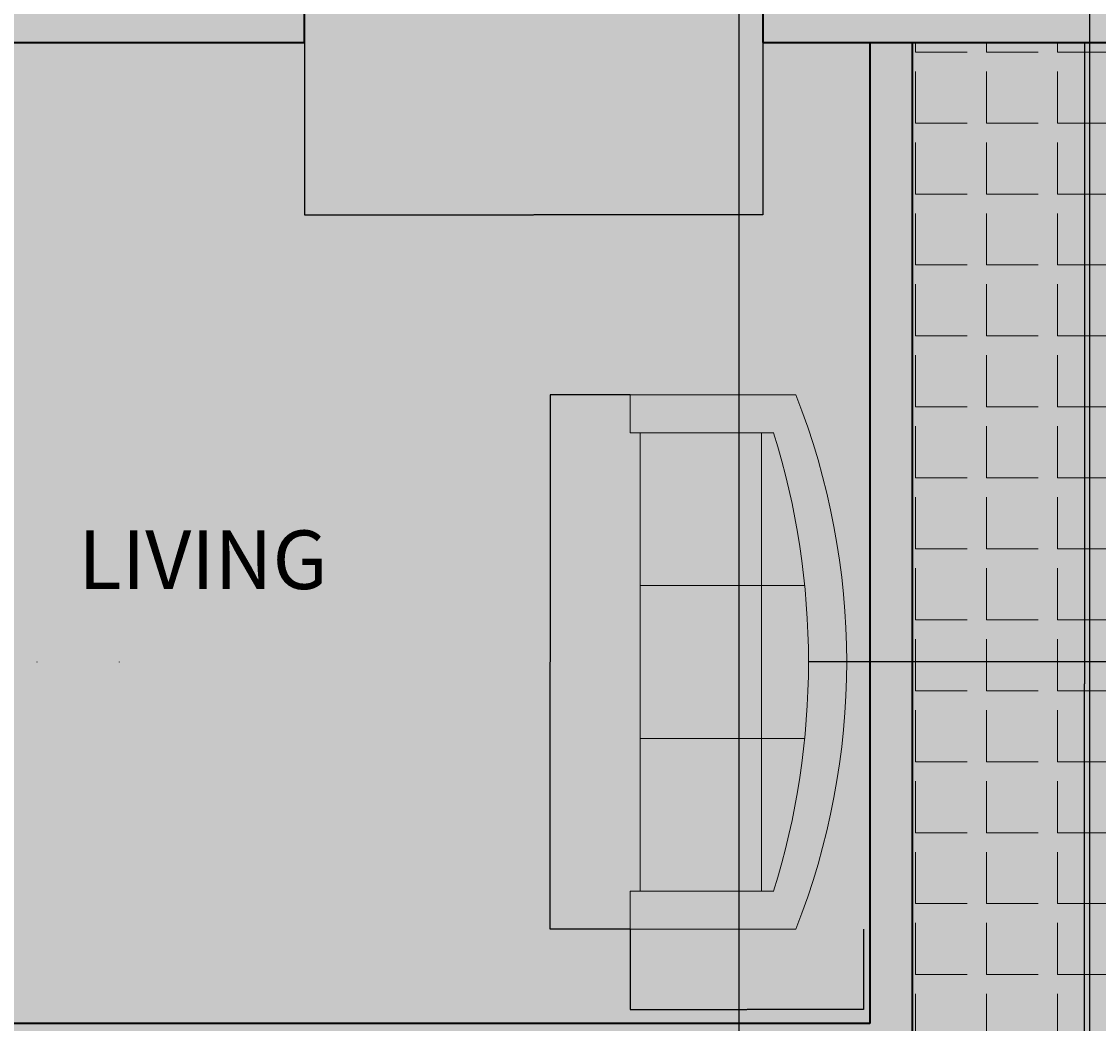
# Model space of a CAD drawing. Units: millimetres. Extents: x 1166 to 16630, y -7192 to 2820.
# Tile 3 of 8: x 2769 to 5842, y -5443 to -2583. Entities that reach past the tile are written whole.
import ezdxf

# ---------------------------------------------------------------- set-up
doc = ezdxf.new("R2010")
doc.units = ezdxf.units.MM
for name, color, linetype, lineweight in [('A-ANNO-DIMS', 2, 'Continuous', 18), ('A-AREA-IDEN', 7, 'Continuous', 18), ('A-FLOR-PATT', 8, 'Continuous', 13), ('A-FURN', 8, 'Continuous', 18), ('A-WALL', 7, 'Continuous', 35)]:
    doc.layers.add(name, color=color, linetype=linetype, lineweight=lineweight)
for name, color, linetype, lineweight, true_color in [('A-FLOR-FNSH-PATT', 254, 'Continuous', 13, 0xfeeab9), ('A-FURN-PATT', 254, 'Continuous', 13, 0xd7c8d7), ('A-WALL-PATT', 254, 'Continuous', 13, 0xcecce6)]:
    doc.layers.add(name, color=color, linetype=linetype, lineweight=lineweight, true_color=true_color)
doc.styles.get("Standard").update_dxf_attribs({"font": 'arial.ttf'})
doc.dimstyles.get("Standard").update_dxf_attribs({"dimtxt": 0.18, "dimasz": 0.18, "dimexe": 0.18, "dimexo": 0.0625, "dimgap": 0.09, "dimtad": 0, "dimtih": 1, "dimtoh": 1, "dimdec": 4, "dimzin": 0, "dimdsep": 46, "dimtxsty": 'Standard', "dimcen": 0.09, "dimadec": 0, "dimazin": 0, "dimtfac": 1, "dimtdec": 4, "dimtofl": 0, "dimtmove": 0, "dimatfit": 3, "dimfxl": 1, "dimtolj": 1, "dimtzin": 0, "dimarcsym": 0})

# ---------------------------------------------------------------- blocks, each defined once
blk = doc.blocks.new('Sofa - Roundback 7 ft.')
for p, q in [((-12.00002, -32.4421), (-12.00003, -6.5971)), ((11.99997, -32.4421), (11.99998, -6.5971)), ((-36.000027, -34), (-36.000027, -11.4696)), ((35.99998, -34), (35.99998, -11.4696)), ((-35.999844, -13.3819), (35.9998, -13.3819)), ((-36.000027, -32.4421), (35.99998, -32.4421))]:
    blk.add_line(p, q)
for points in [[(-36.000027, -34), (-42.000027, -34), (-42.000027, -8)], [(41.99998, -8), (41.99998, -34), (35.99998, -34)]]:
    blk.add_lwpolyline(points)
for centre, radius, start, end in [((0, -114.25), 114.25, 68.43141, 111.5686), ((-0.00001, -127.1968), 121.1968, 72.72033, 107.2797)]:
    blk.add_arc(centre, radius, start, end)
blk = doc.blocks.new('*D21')
at = {"layer": 'A-ANNO-DIMS', "color": 0, "lineweight": -2, "transparency": 16777216}
for p, q in [((4505.6, -3647.9), (4276.6, -3647.9)), ((4276.8, -3648.1), (4276.8, -4410.5)), ((4276.8, -5173.4), (4276.8, -4410.9)), ((4505.6, -5173.5), (4276.6, -5173.5))]:
    blk.add_line(p, q, dxfattribs=at)
at = {"layer": 'A-ANNO-DIMS', "color": 0, "transparency": 16777216}
for points in [[(4276.8, -3648.1), (4276.8, -3648.1), (4276.8, -3647.9)], [(4276.8, -5173.4), (4276.8, -5173.4), (4276.8, -5173.5)]]:
    blk.add_solid(points, dxfattribs=at)
at = {"layer": 'Defpoints', "color": 0, "transparency": 16777216}
for p in [(4505.6, -3647.9), (4276.8, -5173.5), (4505.6, -5173.5)]:
    blk.add_point(p, dxfattribs=at)
at = {"layer": 'A-ANNO-DIMS', "color": 0, "transparency": 16777216, "insert": (4276.8, -4410.7), "char_height": 0.18, "attachment_point": 5}
blk.add_mtext('\\A1;SOFA 1526', dxfattribs=at)
blk = doc.blocks.new('*D22')
at = {"layer": 'A-ANNO-DIMS', "color": 0, "lineweight": -2, "transparency": 16777216}
for p, q in [((4505.6, -5173.6), (4505.6, -5402.6)), ((5171.6, -5173.6), (5171.6, -5402.6)), ((4505.8, -5402.4), (4838.3, -5402.4)), ((5171.4, -5402.4), (4838.9, -5402.4))]:
    blk.add_line(p, q, dxfattribs=at)
at = {"layer": 'A-ANNO-DIMS', "color": 0, "transparency": 16777216}
for points in [[(4505.8, -5402.4), (4505.8, -5402.4), (4505.6, -5402.4)], [(5171.4, -5402.4), (5171.4, -5402.4), (5171.6, -5402.4)]]:
    blk.add_solid(points, dxfattribs=at)
at = {"layer": 'Defpoints', "color": 0, "transparency": 16777216}
for p in [(4505.6, -5173.5), (5171.6, -5173.5), (5171.6, -5402.4)]:
    blk.add_point(p, dxfattribs=at)
at = {"layer": 'A-ANNO-DIMS', "color": 0, "transparency": 16777216, "insert": (4838.6, -5402.4), "char_height": 0.18, "attachment_point": 5}
blk.add_mtext('\\A1;666', dxfattribs=at)
blk = doc.blocks.new('*D36')
at = {"layer": 'A-ANNO-DIMS', "color": 0, "lineweight": -2, "transparency": 16777216}
for p, q in [((4815.9, -849.9), (4815.9, -7065.6)), ((5815.9, -849.9), (5815.9, -7065.6)), ((4816.1, -7065.4), (5315.6, -7065.4)), ((5815.8, -7065.4), (5316.3, -7065.4))]:
    blk.add_line(p, q, dxfattribs=at)
at = {"layer": 'A-ANNO-DIMS', "color": 0, "transparency": 16777216}
for points in [[(4816.1, -7065.4), (4816.1, -7065.5), (4815.9, -7065.4)], [(5815.8, -7065.4), (5815.8, -7065.5), (5815.9, -7065.4)]]:
    blk.add_solid(points, dxfattribs=at)
at = {"layer": 'Defpoints', "color": 0, "transparency": 16777216}
for p in [(4815.9, -849.8), (5815.9, -849.8), (5815.9, -7065.4)]:
    blk.add_point(p, dxfattribs=at)
at = {"layer": 'A-ANNO-DIMS', "color": 0, "transparency": 16777216, "insert": (5315.9, -7065.4), "char_height": 0.18, "attachment_point": 5}
blk.add_mtext('\\A1;1000', dxfattribs=at)
blk = doc.blocks.new('*D39')
at = {"layer": 'A-ANNO-DIMS', "color": 0, "lineweight": -2, "transparency": 16777216}
for p, q in [((5309.7, -2642.5), (5801.8, -2642.5)), ((5801.6, -2642.7), (5801.6, -4473.2)), ((5801.6, -6304), (5801.6, -4473.5)), ((5309.7, -6304.1), (5801.8, -6304.1))]:
    blk.add_line(p, q, dxfattribs=at)
at = {"layer": 'A-ANNO-DIMS', "color": 0, "transparency": 16777216}
for points in [[(5801.6, -2642.7), (5801.6, -2642.7), (5801.6, -2642.5)], [(5801.6, -6304), (5801.6, -6304), (5801.6, -6304.1)]]:
    blk.add_solid(points, dxfattribs=at)
at = {"layer": 'Defpoints', "color": 0, "transparency": 16777216}
for p in [(5309.6, -2642.5), (5309.6, -6304.1), (5801.6, -6304.1)]:
    blk.add_point(p, dxfattribs=at)
at = {"layer": 'A-ANNO-DIMS', "color": 0, "transparency": 16777216, "insert": (5801.6, -4473.3), "char_height": 0.18, "attachment_point": 5}
blk.add_mtext('\\A1;3661.6', dxfattribs=at)
blk = doc.blocks.new('*D47')
at = {"layer": 'A-ANNO-DIMS', "color": 0, "lineweight": -2, "transparency": 16777216}
for p, q in [((3575.9, -2642.6), (3575.9, -3134.7)), ((4884, -2642.6), (4884, -3134.7)), ((3576.1, -3134.5), (4229.6, -3134.5)), ((4883.8, -3134.5), (4230.3, -3134.5))]:
    blk.add_line(p, q, dxfattribs=at)
at = {"layer": 'A-ANNO-DIMS', "color": 0, "transparency": 16777216}
for points in [[(3576.1, -3134.5), (3576.1, -3134.6), (3575.9, -3134.5)], [(4883.8, -3134.5), (4883.8, -3134.6), (4884, -3134.5)]]:
    blk.add_solid(points, dxfattribs=at)
at = {"layer": 'Defpoints', "color": 0, "transparency": 16777216}
for p in [(3575.9, -2642.5), (4884, -2642.5), (3575.9, -3134.5)]:
    blk.add_point(p, dxfattribs=at)
at = {"layer": 'A-ANNO-DIMS', "color": 0, "transparency": 16777216, "insert": (4230, -3134.5), "char_height": 0.18, "attachment_point": 5}
blk.add_mtext('\\A1;1308', dxfattribs=at)
blk = doc.blocks.new('*D69')
at = {"layer": 'A-ANNO-DIMS', "color": 0, "lineweight": -2, "transparency": 16777216}
for p, q in [((2812.8, -4410.7), (2813, -4410.7)), ((2812.9, -4410.8), (2812.9, -4410.6)), ((6334.9, -4410.7), (5014.4, -4410.7))]:
    blk.add_line(p, q, dxfattribs=at)
at = {"layer": 'A-ANNO-DIMS', "color": 0, "transparency": 16777216}
blk.add_solid([(5014.4, -4410.7), (5014.4, -4410.7), (5014.2, -4410.7)], dxfattribs=at)
at = {"layer": 'Defpoints', "color": 0, "transparency": 16777216}
for p in [(2812.9, -4410.7), (5014.2, -4410.7)]:
    blk.add_point(p, dxfattribs=at)
at = {"layer": 'A-ANNO-DIMS', "color": 0, "transparency": 16777216, "insert": (6335.5, -4410.7), "char_height": 0.18, "attachment_point": 5}
blk.add_mtext('\\A1;R2201.3', dxfattribs=at)
blk = doc.blocks.new('*D70')
at = {"layer": 'A-ANNO-DIMS', "color": 0, "lineweight": -2, "transparency": 16777216}
for p, q in [((3048, -4410.7), (3048.2, -4410.7)), ((3048.1, -4410.8), (3048.1, -4410.6)), ((6368.2, -4410.7), (5123.3, -4410.7))]:
    blk.add_line(p, q, dxfattribs=at)
at = {"layer": 'A-ANNO-DIMS', "color": 0, "transparency": 16777216}
blk.add_solid([(5123.3, -4410.7), (5123.3, -4410.7), (5123.2, -4410.7)], dxfattribs=at)
at = {"layer": 'Defpoints', "color": 0, "transparency": 16777216}
for p in [(3048.1, -4410.7), (5123.2, -4410.7)]:
    blk.add_point(p, dxfattribs=at)
at = {"layer": 'A-ANNO-DIMS', "color": 0, "transparency": 16777216, "insert": (6368.7, -4410.7), "char_height": 0.18, "attachment_point": 5}
blk.add_mtext('\\A1;R2075', dxfattribs=at)

msp = doc.modelspace()

# ---------------------------------------------------------------- hatches: boundary and pattern name
at = {"layer": 'A-FLOR-FNSH-PATT', "transparency": 33554523}
h = msp.add_hatch(color=256, dxfattribs=at)
h.dxf.hatch_style = 1
h.paths.add_polyline_path([(7725.939, 2327.462), (1725.939, 2327.462), (1725.939, -5672.538), (5309.615, -5672.538), (5309.615, -2642.538), (5189.615, -2642.538), (5189.615, -5442.538), (1955.939, -5442.538), (1955.939, 2097.462), (4665.939, 2097.462), (4665.939, 150.2), (4815.939, 150.2, -0.40145271), (5814.982, -806.05), (5815.939, -806.05), (5815.939, -849.8), (4815.939, -849.8), (4785.939, -849.8), (4785.939, -902.538), (7495.939, -902.538), (7495.939, -2522.538), (4884.014, -2522.538), (4884.014, -2642.538), (7725.939, -2642.538)], flags=17)
h.paths.add_polyline_path([(6066.077, 618.421), (6066.077, 1624.186), (7407.098, 1624.186), (7407.098, 618.421)], flags=16)
h.paths.add_polyline_path([(4979.212, 660.219), (4799.278, 660.219), (4799.278, 780.174), (4789.282, 790.171), (4789.282, 870.141), (4799.278, 880.137), (4799.278, 1259.997), (4979.212, 1259.997), (4979.212, 1230.008), (4989.208, 1230.008), (4989.208, 1110.052), (4979.212, 1110.052), (4979.212, 1100.056), (4989.208, 1100.056), (4989.208, 980.1), (4979.212, 980.1), (4979.212, 950.111), (4989.208, 950.111), (4989.208, 940.115, -0.09090909), (4989.208, 720.196), (4989.208, 710.2), (4979.212, 710.2)], flags=16)
h.paths.add_polyline_path([(4974.214, 665.217), (4804.276, 665.217), (4804.276, 1254.999), (4974.214, 1254.999)], flags=0)
h.paths.add_polyline_path([(6910.92, 618.421), (6910.92, 873.215), (7165.714, 873.215), (7165.714, 1490.084), (7386.983, 1490.084), (7386.983, 1141.419), (7165.714, 1141.419), (7165.714, 1101.188), (7386.983, 1101.188), (7386.983, 752.523), (7132.189, 752.523), (7132.189, 839.689)], flags=16)
h.paths.add_polyline_path([(4815.939, 150.2), (4665.939, 150.2), (4665.939, 1500.697), (2460.545, 1500.697), (2460.545, -402.538), (3575.939, -402.538), (3575.939, -1706.64), (3463.439, -1706.64, 0.40145271), (2714.158, -2423.828), (3463.439, -2423.828), (3463.439, -2456.64), (3455.939, -2522.538), (3455.939, -2456.64), (2713.439, -2456.64), (2713.439, -2423.828), (2714.158, -2423.828, -0.39855266), (3455.939, -1706.678), (3455.939, -1706.64), (3575.939, -1706.64), (3575.939, -402.538), (2460.545, -402.538), (2460.545, 1500.697), (4665.939, 1500.697), (4665.939, 150.2), (4785.939, 150.2), (4785.939, 2097.462), (7495.939, 2097.462), (7495.939, -2522.538), (4884.014, -2522.538), (4884.014, -2642.538), (7725.939, -2642.538), (7725.939, 2327.462), (1725.939, 2327.462), (1725.939, -5672.538), (5309.615, -5672.538), (5309.615, -2642.538), (4884.014, -2642.538), (4884.014, -2522.538), (4884.014, -1822.538), (4665.939, -1822.538), (4665.939, -1722.538), (4665.939, -1022.538), (4665.939, -849.8), (4815.939, -849.8), (4815.939, -806.05), (5814.982, -806.05, 0.40145271)])
h.paths.add_polyline_path([(1955.939, -4323.626), (1965.936, -4313.63), (1965.936, -3933.77), (2145.869, -3933.77), (2145.869, -3963.759), (2155.866, -3963.759), (2155.866, -4083.715), (2145.869, -4083.715), (2145.869, -4093.711), (2155.866, -4093.711), (2155.866, -4213.667), (2145.869, -4213.667), (2145.869, -4243.656), (2155.866, -4243.656), (2155.866, -4253.652, -0.09090909), (2155.866, -4473.571), (2155.866, -4483.567), (2145.869, -4483.567), (2145.869, -4533.549), (1965.936, -4533.549), (1965.936, -4413.593), (1955.939, -4403.597)], flags=16)
h.paths.add_polyline_path([(3017.672, -1268.685), (3017.672, -1558.932), (2092.538, -1558.932), (2092.538, -1268.685)], flags=16)
h.paths.add_polyline_path([(2768.799, -687.028), (2664.904, -687.028), (2696.871, -782.93, -0.50132349), (2617.667, -1084.405, -0.13289091), (2584.271, -1084.405, -0.50131678), (2505.065, -782.933), (2537.033, -687.028), (2489.082, -687.028), (2489.082, -711.004), (2441.13, -711.004), (2441.13, -687.028), (2433.138, -687.028), (2433.138, -559.158), (2768.799, -559.158)], flags=16)
h.paths.add_polyline_path([(2752.815, -655.061, -0.41421356), (2740.827, -671.045), (2465.106, -671.045, -0.41421356), (2449.122, -659.057), (2449.122, -591.126, -0.41421356), (2461.11, -575.142), (2736.831, -575.142, -0.41421356), (2752.815, -587.13)], flags=0)
h.paths.add_polyline_path([(2627.247, -1063.016, -0.21500378), (2574.691, -1063.016, -0.48007965), (2537.034, -782.931), (2664.904, -782.931, -0.4800795)], flags=0)
h.paths.add_polyline_path([(4505.634, -3647.875), (4977.863, -3647.875, -0.19047621), (4977.864, -5173.541), (4505.634, -5173.541), (4505.634, -5064.565), (4533.929, -5064.565), (4533.929, -3756.851), (4505.634, -3756.851)], flags=16)
h.paths.add_polyline_path([(4880.114, -4192.756), (5003.372, -4192.756, -0.04962821), (5003.372, -4628.66), (4880.114, -4628.66)], flags=0)
h.paths.add_polyline_path([(2140.871, -3938.769), (2140.871, -4528.551), (1970.934, -4528.551), (1970.934, -3938.769)], flags=0)
h.paths.add_polyline_path([(7495.939, -1022.538), (6660.699, -1022.538), (6660.699, -1722.538, -0.21291191), (6697.901, -1739.132)], flags=16)
h.paths.add_polyline_path([(7495.939, -1022.538), (6697.901, -1739.132, -0.18498743), (6710.699, -1772.538), (7495.939, -1772.538)], flags=16)
h.paths.add_polyline_path([(7495.939, -1772.538), (6710.699, -1772.538, -0.18498743), (6697.901, -1805.944), (7495.939, -2522.538)], flags=16)
h.paths.add_polyline_path([(6697.901, -1805.944, -0.21291191), (6660.699, -1822.538), (6660.699, -2522.538), (7495.939, -2522.538)], flags=16)
h.paths.add_polyline_path([(6660.699, -1822.538), (6438.613, -1822.538), (6438.613, -2522.538), (6660.699, -2522.538)], flags=16)
h.paths.add_polyline_path([(6438.613, -1822.538), (6216.528, -1822.538), (6216.528, -2522.538), (6438.613, -2522.538)], flags=16)
h.paths.add_polyline_path([(6216.528, -1822.538), (5994.442, -1822.538), (5994.442, -2522.538), (6216.528, -2522.538)], flags=16)
h.paths.add_polyline_path([(5994.442, -1822.538), (5772.357, -1822.538), (5772.357, -2522.538), (5994.442, -2522.538)], flags=16)
h.paths.add_polyline_path([(5550.271, -1822.538), (5328.185, -1822.538), (5328.185, -2522.538), (5550.271, -2522.538)], flags=16)
h.paths.add_polyline_path([(5328.185, -1822.538), (5106.1, -1822.538), (5106.1, -2522.538), (5328.185, -2522.538)], flags=16)
h.paths.add_polyline_path([(5106.1, -1822.538), (4884.014, -1822.538), (4884.014, -2522.538), (5106.1, -2522.538)], flags=16)
h.paths.add_polyline_path([(4884.014, -1022.538), (4665.939, -1022.538), (4665.939, -1722.538), (4884.014, -1722.538)], flags=16)
h.paths.add_polyline_path([(5106.1, -1022.538), (4884.014, -1022.538), (4884.014, -1722.538), (5106.1, -1722.538)], flags=16)
h.paths.add_polyline_path([(5550.271, -1022.538), (5328.185, -1022.538), (5328.185, -1722.538), (5550.271, -1722.538)], flags=16)
h.paths.add_polyline_path([(5328.185, -1022.538), (5106.1, -1022.538), (5106.1, -1722.538), (5328.185, -1722.538)], flags=16)
h.paths.add_polyline_path([(5772.357, -1022.538), (5550.271, -1022.538), (5550.271, -1722.538), (5772.357, -1722.538)], flags=16)
h.paths.add_polyline_path([(5994.442, -1022.538), (5772.357, -1022.538), (5772.357, -1722.538), (5994.442, -1722.538)], flags=16)
h.paths.add_polyline_path([(6216.528, -1022.538), (5994.442, -1022.538), (5994.442, -1722.538), (6216.528, -1722.538)], flags=16)
h.paths.add_polyline_path([(6660.699, -1022.538), (6438.613, -1022.538), (6438.613, -1722.538), (6660.699, -1722.538)], flags=16)
h.paths.add_polyline_path([(6438.613, -1022.538), (6216.528, -1022.538), (6216.528, -1722.538), (6438.613, -1722.538)], flags=16)
h.paths.add_polyline_path([(5772.357, -1822.538), (5550.271, -1822.538), (5550.271, -2522.538), (5772.357, -2522.538)], flags=16)
h.paths.add_polyline_path([(6660.699, -1722.538), (6438.613, -1722.538), (4665.939, -1722.538), (4665.939, -1822.538), (6660.699, -1822.538, 0.21291191), (6697.901, -1805.944, 0.64892437)], flags=16)
h.paths.add_polyline_path([(5860.25, -44.006), (7154.504, -44.006), (7154.504, 215.689), (5860.25, 215.689)], flags=24)
h.paths.add_polyline_path([(2102.336, -1543.656), (3007.075, -1543.656), (3007.075, -1283.961), (2102.336, -1283.961)], flags=8)
h.paths.add_polyline_path([(2887.503, -4248.68), (3740.372, -4248.68), (3740.372, -3989.156), (2887.503, -3989.156)], flags=24)
h.paths.add_polyline_path([(2999.436, 433.054), (4111.829, 433.054), (4111.829, 692.578), (2999.436, 692.578)], flags=24)
at = {"layer": 'A-FLOR-FNSH-PATT', "transparency": 33554590}
h = msp.add_hatch(color=256, dxfattribs=at)
h.dxf.hatch_style = 1
h.paths.add_polyline_path([(5309.615, -2642.538), (5309.615, -6304.141), (7725.939, -6304.141), (7725.939, -5672.538), (7725.939, -2642.538)])
edge = h.paths.add_edge_path(flags=16)
edge.add_ellipse((-448.972, -3645.43), major_axis=(-7430.723, 0), ratio=0.84230387, start_angle=182.1799503, end_angle=183.6504276, ccw=False)
edge.add_line((6974.174, -3362.862), (6984.716, -3362.862))
edge.add_ellipse((6982.281, -3380.397), major_axis=(-20.817, 0), ratio=0.84230387, start_angle=180, end_angle=270, ccw=False)
edge.add_line((7003.098, -3380.397), (7003.098, -3722.916))
edge.add_ellipse((6982.281, -3720.865), major_axis=(20.817, 0), ratio=0.84230387, start_angle=270, end_angle=360, ccw=False)
edge.add_ellipse((-142030.923, -3973.064), major_axis=(149013.204, 0), ratio=0.8423038695, start_angle=-0.38386678, end_angle=0.09022909, ccw=False)
edge.add_line((6977.567, -4971.397), (6984.47, -4971.397))
edge.add_ellipse((6982.281, -4988.932), major_axis=(20.817, 0), ratio=0.84230387, start_angle=0, end_angle=90, ccw=False)
edge.add_line((7003.098, -4988.932), (7003.098, -5331.243))
edge.add_ellipse((6982.281, -5329.4), major_axis=(-20.817, 0), ratio=0.84230387, start_angle=90, end_angle=180, ccw=False)
edge.add_line((6982.281, -5346.934), (6973.354, -5346.934))
edge.add_ellipse((-142030.923, -3973.064), major_axis=(149013.204, 0), ratio=0.8423038695, start_angle=-0.6186432, end_angle=-0.52827147, ccw=False)
edge.add_ellipse((6960.189, -5606.903), major_axis=(-31.226, 0), ratio=0.84230387, start_angle=179.371763, end_angle=248.464757, ccw=False)
edge.add_ellipse((-142041.332, -3973.064), major_axis=(-149045.372, 0), ratio=0.8423038661, start_angle=179.35344592, end_angle=179.3717628, ccw=False)
edge.add_ellipse((6916.87, -5654.054), major_axis=(-73.802, 0), ratio=0.84230387, start_angle=90, end_angle=179.353446, ccw=False)
edge.add_line((6916.87, -5716.218), (5995.23, -5716.218))
edge.add_ellipse((5995.23, -5654.054), major_axis=(73.802, 0), ratio=0.84230387, start_angle=180.646554, end_angle=270, ccw=False)
edge.add_ellipse((154953.432, -3973.064), major_axis=(-149045.372, 0), ratio=0.8423038697, start_angle=0.62823722, end_angle=0.6465541, ccw=False)
edge.add_ellipse((5951.911, -5606.903), major_axis=(31.226, 0), ratio=0.84230387, start_angle=111.535244, end_angle=180.628237, ccw=False)
edge.add_ellipse((154943.023, -3973.064), major_axis=(-149013.204, 0), ratio=0.8423038695, start_angle=0.52827147, end_angle=0.6465541, ccw=False)
edge.add_line((5938.746, -5346.934), (5927.384, -5346.934))
edge.add_ellipse((5929.819, -5329.4), major_axis=(20.817, 0), ratio=0.84230387, start_angle=180, end_angle=270, ccw=False)
edge.add_line((5909.002, -5329.4), (5909.002, -4986.881))
edge.add_ellipse((5929.819, -4988.932), major_axis=(-20.817, 0), ratio=0.84230387, start_angle=-90, end_angle=0, ccw=False)
edge.add_line((5929.819, -4971.397), (5934.533, -4971.397))
edge.add_ellipse((154943.023, -3973.064), major_axis=(-149013.204, 0), ratio=0.8423038695, start_angle=-0.09022909, end_angle=0.38386678, ccw=False)
edge.add_ellipse((5929.819, -3720.865), major_axis=(-20.817, 0), ratio=0.84230387, start_angle=0, end_angle=90, ccw=False)
edge.add_line((5909.002, -3720.865), (5909.002, -3378.346))
edge.add_ellipse((5929.819, -3380.397), major_axis=(20.817, 0), ratio=0.84230387, start_angle=90, end_angle=180, ccw=False)
edge.add_line((5929.819, -3362.862), (5937.926, -3362.862))
edge.add_ellipse((13361.072, -3645.43), major_axis=(7430.723, 0), ratio=0.84230387, start_angle=176.3495724, end_angle=177.8200497, ccw=False)
edge.add_ellipse((6843.239, -6808.261), major_axis=(4407.333, 0), ratio=0.84230387, start_angle=102.125966, end_angle=103.780529, ccw=False)
edge.add_ellipse((6843.239, -6711.831), major_axis=(4294.728, 0), ratio=0.84230387, start_angle=100.209539, end_angle=102.444627, ccw=False)
edge.add_ellipse((5718.978, -189.342), major_axis=(-3530.283, 0), ratio=0.84230387, start_angle=99.256566, end_angle=102.554933)
edge.add_line((6369.843, -3111.939), (6452.047, -3066.483))
edge.add_ellipse((6456.05, -3074.757), major_axis=(-10.409, 0), ratio=0.84230387, start_angle=270, end_angle=307.93313, ccw=False)
edge.add_ellipse((6456.05, -3074.757), major_axis=(-10.409, 0), ratio=0.84230387, start_angle=232.06687, end_angle=270, ccw=False)
edge.add_line((6461.762, -3067.428), (6542.257, -3111.939))
edge.add_ellipse((7193.122, -189.342), major_axis=(3530.283, 0), ratio=0.84230387, start_angle=257.445067, end_angle=260.743434)
edge.add_ellipse((6068.861, -6711.831), major_axis=(4294.728, 0), ratio=0.84230387, start_angle=77.555373, end_angle=79.790461, ccw=False)
edge.add_ellipse((6068.861, -6808.261), major_axis=(-4407.333, 0), ratio=0.84230387, start_angle=256.219471, end_angle=257.874034, ccw=False)
edge = h.paths.add_edge_path(flags=0)
edge.add_ellipse((5799.636, -3484.806), major_axis=(790.133, 0), ratio=0.84230387, start_angle=0, end_angle=29.43857, ccw=False)
edge.add_line((6589.77, -3484.806), (6589.77, -3517.866))
edge.add_line((6589.77, -3517.866), (6615.397, -3517.866))
edge.add_ellipse((6612.95, -3526.633), major_axis=(10.409, 0), ratio=0.84230387, start_angle=45.519789, end_angle=90, ccw=False)
edge.add_line((6619.584, -3519.877), (6697.577, -3574.216))
edge.add_line((6697.577, -3574.216), (6697.577, -3782.552))
edge.add_ellipse((6643.673, -3780.461), major_axis=(5.016, 89.187), ratio=0.60383358, start_angle=106.342592, end_angle=270.997986, ccw=False)
edge.add_line((6589.77, -3793.028), (6589.77, -3484.806))
edge.add_ellipse((5799.636, -3484.806), major_axis=(790.133, 0), ratio=0.84230387, start_angle=0, end_angle=29.43857)
edge.add_ellipse((7112.464, -3484.806), major_axis=(-790.133, 0), ratio=0.84230387, start_angle=-29.43857, end_angle=0)
edge.add_line((6322.33, -3484.806), (6322.33, -3793.028))
edge.add_ellipse((6268.427, -3780.461), major_axis=(-5.016, 89.187), ratio=0.60383358, start_angle=89.002014, end_angle=253.657408, ccw=False)
edge.add_line((6214.523, -3782.552), (6214.523, -3574.216))
edge.add_line((6214.523, -3574.216), (6294.401, -3518.564))
edge.add_ellipse((6299.15, -3526.633), major_axis=(10.409, 0), ratio=0.84230387, start_angle=90, end_angle=134.480211, ccw=False)
edge.add_line((6299.15, -3517.866), (6322.33, -3517.866))
edge.add_line((6322.33, -3517.866), (6322.33, -3484.806))
edge.add_ellipse((7112.464, -3484.806), major_axis=(-790.133, 0), ratio=0.84230387, start_angle=-29.43857, end_angle=0, ccw=False)
edge = h.paths.add_edge_path(flags=0)
edge.add_line((6899.672, -4051.113), (6868.937, -4281.474))
edge.add_ellipse((6495.43, -5170.363), major_axis=(1119.455, 0), ratio=0.84230387, start_angle=67.208085, end_angle=85.12993)
edge.add_line((6575.565, -4229.86), (6336.535, -4229.86))
edge.add_ellipse((6416.67, -5170.363), major_axis=(1119.455, 0), ratio=0.84230387, start_angle=94.87007, end_angle=112.791915)
edge.add_line((6043.163, -4281.474), (6012.428, -4051.113))
edge.add_ellipse((6380.264, -4969.144), major_axis=(1150.303, 0), ratio=0.84230387, start_angle=94.277421, end_angle=111.834954, ccw=False)
edge.add_line((6307.939, -4002.156), (6604.161, -4002.156))
edge.add_ellipse((6531.836, -4969.144), major_axis=(-1150.303, 0), ratio=0.84230387, start_angle=248.165046, end_angle=265.722579, ccw=False)
edge = h.paths.add_edge_path(flags=0)
edge.add_ellipse((-142030.923, -3973.064), major_axis=(-148992.387, 0), ratio=0.8423038695, start_angle=179.62223581, end_angle=179.94440569, ccw=False)
edge.add_line((6956.9, -4955.389), (6903.068, -4744.03))
edge.add_ellipse((-45118.924, -4413.46), major_axis=(52023.473, 0), ratio=0.84230387, start_angle=-0.3640763, end_angle=0.1208974)
edge.add_line((6904.386, -4303.688), (6961.365, -4117.632))
edge = h.paths.add_edge_path(flags=0)
edge.add_line((5950.735, -4117.632), (6007.714, -4303.688))
edge.add_ellipse((58031.024, -4413.46), major_axis=(-52023.473, 0), ratio=0.84230387, start_angle=-0.1208974, end_angle=0.3640763)
edge.add_line((6009.031, -4744.03), (5955.2, -4955.389))
edge.add_ellipse((154943.023, -3973.064), major_axis=(-148992.387, 0), ratio=0.8423038696, start_angle=0.05559431, end_angle=0.37776419, ccw=False)
edge = h.paths.add_edge_path(flags=0)
edge.add_line((6868.937, -5013.198), (6868.937, -5277.993))
edge.add_ellipse((6456.05, -3571.079), major_axis=(2068.116, 0), ratio=0.84230387, start_angle=256.401865, end_angle=283.598135, ccw=False)
edge.add_line((6043.163, -5277.993), (6043.163, -5013.198))
edge.add_ellipse((6456.05, -3306.285), major_axis=(2068.116, 0), ratio=0.84230387, start_angle=256.401865, end_angle=283.598135)
edge = h.paths.add_edge_path(flags=0)
edge.add_ellipse((6827.303, -5415.313), major_axis=(-41.634, 0), ratio=0.84230387, start_angle=180, end_angle=270, ccw=False)
edge.add_line((6868.937, -5415.313), (6868.937, -5689.123))
edge.add_line((6868.937, -5689.123), (6043.163, -5689.123))
edge.add_line((6043.163, -5689.123), (6043.163, -5415.313))
edge.add_ellipse((6084.797, -5415.313), major_axis=(-41.634, 0), ratio=0.84230387, start_angle=-90, end_angle=0, ccw=False)
edge.add_line((6084.797, -5380.245), (6827.303, -5380.245))
h.paths.add_polyline_path([(3455.939, -522.538), (1955.939, -522.538), (1955.939, -2522.538), (3455.939, -2522.538), (3455.939, -2456.64), (2713.439, -2456.64), (2713.439, -2423.828), (2714.158, -2423.828, -0.39855266), (3455.939, -1706.678)])
h.paths.add_polyline_path([(2617.667, -1084.405, -0.13289091), (2584.271, -1084.405, -0.50131678), (2505.065, -782.933), (2537.033, -687.028), (2489.082, -687.028), (2489.082, -711.004), (2441.13, -711.004), (2441.13, -695.02), (2473.098, -695.02), (2473.098, -687.028), (2433.138, -687.028), (2433.138, -559.158), (2768.799, -559.158), (2768.799, -687.028), (2664.904, -687.028), (2696.871, -782.93, -0.50132349)], flags=16)
h.paths.add_polyline_path([(2627.247, -1063.016, -0.21500378), (2574.691, -1063.016, -0.48007965), (2537.034, -782.931), (2664.904, -782.931, -0.4800795)], flags=0)
h.paths.add_polyline_path([(2736.831, -671.045), (2465.106, -671.045, -0.50000012), (2449.122, -655.061), (2449.122, -591.126, -0.50000012), (2465.106, -575.142), (2736.831, -575.142, -0.50000012), (2752.815, -591.126), (2752.815, -655.061, -0.50000012)], flags=0)
h.paths.add_polyline_path([(5931.782, -6111.826), (7070.31, -6111.826), (7070.31, -5852.302), (5931.782, -5852.302)], flags=24)
h.paths.add_polyline_path([(2102.336, -1543.656), (3007.075, -1543.656), (3007.075, -1283.961), (2102.336, -1283.961)], flags=24)
at = {"layer": 'A-FLOR-PATT', "transparency": 33554564}
h = msp.add_hatch(dxfattribs=at)
h.set_pattern_fill('ANGLE', color=256, scale=29)
h.set_pattern_definition([(0, (-8657.52, -11987.85), (0, 202.565), [147.32, -55.245]), (90, (-8657.52, -11987.85), (-202.565, 1e-14), [147.32, -55.245])])
h.paths.add_polyline_path([(7725.939, -2642.538), (5309.615, -2642.538), (5309.615, -6304.141), (7725.939, -6304.141), (7725.939, -5672.538)])
edge = h.paths.add_edge_path(flags=16)
edge.add_ellipse((-142030.923, -3973.064), major_axis=(149013.204, 0), ratio=0.8423038695, start_angle=-0.38386678, end_angle=0.09022909, ccw=False)
edge.add_ellipse((6982.281, -4988.932), major_axis=(20.817, 0), ratio=0.84230387, start_angle=0, end_angle=90, ccw=False)
edge.add_line((7003.098, -4988.932), (7003.098, -5329.4))
edge.add_ellipse((6982.281, -5329.4), major_axis=(-20.817, 0), ratio=0.84230387, start_angle=90, end_angle=180, ccw=False)
edge.add_line((6982.281, -5346.934), (6973.354, -5346.934))
edge.add_ellipse((-142030.923, -3973.064), major_axis=(149013.204, 0), ratio=0.8423038695, start_angle=-0.6186432, end_angle=-0.52827147, ccw=False)
edge.add_ellipse((6960.189, -5606.903), major_axis=(-31.226, 0), ratio=0.84230387, start_angle=179.371763, end_angle=248.464757, ccw=False)
edge.add_ellipse((-142041.332, -3973.064), major_axis=(-149045.372, 0), ratio=0.8423038661, start_angle=179.35344592, end_angle=179.3717628, ccw=False)
edge.add_ellipse((6916.87, -5654.054), major_axis=(-73.802, 0), ratio=0.84230387, start_angle=90, end_angle=179.353446, ccw=False)
edge.add_line((6916.87, -5716.218), (5995.23, -5716.218))
edge.add_ellipse((5995.23, -5654.054), major_axis=(73.802, 0), ratio=0.84230387, start_angle=180.646554, end_angle=270, ccw=False)
edge.add_ellipse((154953.432, -3973.064), major_axis=(-149045.372, 0), ratio=0.8423038697, start_angle=0.62823722, end_angle=0.6465541, ccw=False)
edge.add_ellipse((5951.911, -5606.903), major_axis=(31.226, 0), ratio=0.84230387, start_angle=111.535244, end_angle=180.628237, ccw=False)
edge.add_ellipse((154943.023, -3973.064), major_axis=(-149013.204, 0), ratio=0.8423038695, start_angle=0.52827147, end_angle=0.6465541, ccw=False)
edge.add_line((5938.746, -5346.934), (5929.819, -5346.934))
edge.add_ellipse((5929.819, -5329.4), major_axis=(20.817, 0), ratio=0.84230387, start_angle=180, end_angle=270, ccw=False)
edge.add_line((5909.002, -5329.4), (5909.002, -4988.932))
edge.add_ellipse((5929.819, -4988.932), major_axis=(-20.817, 0), ratio=0.84230387, start_angle=-90, end_angle=0, ccw=False)
edge.add_ellipse((154943.023, -3973.064), major_axis=(-149013.204, 0), ratio=0.8423038695, start_angle=-0.09022909, end_angle=0.38386678, ccw=False)
edge.add_ellipse((5929.819, -3720.865), major_axis=(-20.817, 0), ratio=0.84230387, start_angle=0, end_angle=90, ccw=False)
edge.add_line((5909.002, -3720.865), (5909.002, -3380.397))
edge.add_ellipse((5929.819, -3380.397), major_axis=(20.817, 0), ratio=0.84230387, start_angle=90, end_angle=180, ccw=False)
edge.add_line((5929.819, -3362.862), (5937.926, -3362.862))
edge.add_ellipse((13361.072, -3645.43), major_axis=(7430.723, 0), ratio=0.84230387, start_angle=176.3495724, end_angle=177.8200497, ccw=False)
edge.add_ellipse((6843.239, -6808.261), major_axis=(4407.333, 0), ratio=0.84230387, start_angle=102.125966, end_angle=103.780529, ccw=False)
edge.add_ellipse((6843.239, -6711.831), major_axis=(4294.728, 0), ratio=0.84230387, start_angle=100.209539, end_angle=102.444627, ccw=False)
edge.add_ellipse((5718.978, -189.342), major_axis=(-3530.283, 0), ratio=0.84230387, start_angle=99.256566, end_angle=102.554933)
edge.add_line((6369.843, -3111.939), (6453.506, -3065.676))
edge.add_ellipse((6456.05, -3074.757), major_axis=(-10.409, 0), ratio=0.84230387, start_angle=232.06687, end_angle=270, ccw=False)
edge.add_line((6460.053, -3066.483), (6542.257, -3111.939))
edge.add_ellipse((7193.122, -189.342), major_axis=(3530.283, 0), ratio=0.84230387, start_angle=257.445067, end_angle=260.743434)
edge.add_ellipse((6068.861, -6711.831), major_axis=(4294.728, 0), ratio=0.84230387, start_angle=77.555373, end_angle=79.790461, ccw=False)
edge.add_ellipse((6068.861, -6808.261), major_axis=(-4407.333, 0), ratio=0.84230387, start_angle=256.219471, end_angle=257.874034, ccw=False)
edge.add_ellipse((-448.972, -3645.43), major_axis=(-7430.723, 0), ratio=0.84230387, start_angle=182.1799503, end_angle=183.6504276, ccw=False)
edge.add_line((6974.174, -3362.862), (6982.281, -3362.862))
edge.add_ellipse((6982.281, -3380.397), major_axis=(-20.817, 0), ratio=0.84230387, start_angle=180, end_angle=270, ccw=False)
edge.add_line((7003.098, -3380.397), (7003.098, -3720.865))
edge.add_ellipse((6982.281, -3720.865), major_axis=(20.817, 0), ratio=0.84230387, start_angle=270, end_angle=360, ccw=False)
edge = h.paths.add_edge_path(flags=0)
edge.add_ellipse((-142030.923, -3973.064), major_axis=(-148992.387, 0), ratio=0.8423038695, start_angle=179.62223581, end_angle=179.94440569, ccw=False)
edge.add_line((6956.9, -4955.389), (6903.068, -4744.03))
edge.add_ellipse((-45118.924, -4413.46), major_axis=(52023.473, 0), ratio=0.84230387, start_angle=-0.3640763, end_angle=0.1208974)
edge.add_line((6904.386, -4303.688), (6961.365, -4117.632))
edge = h.paths.add_edge_path(flags=0)
edge.add_line((6899.672, -4051.113), (6868.937, -4281.474))
edge.add_ellipse((6495.43, -5170.363), major_axis=(1119.455, 0), ratio=0.84230387, start_angle=67.208085, end_angle=85.12993)
edge.add_line((6575.565, -4229.86), (6336.535, -4229.86))
edge.add_ellipse((6416.67, -5170.363), major_axis=(1119.455, 0), ratio=0.84230387, start_angle=94.87007, end_angle=112.791915)
edge.add_line((6043.163, -4281.474), (6012.428, -4051.113))
edge.add_ellipse((6380.264, -4969.144), major_axis=(1150.303, 0), ratio=0.84230387, start_angle=94.277421, end_angle=111.834954, ccw=False)
edge.add_line((6307.939, -4002.156), (6604.161, -4002.156))
edge.add_ellipse((6531.836, -4969.144), major_axis=(-1150.303, 0), ratio=0.84230387, start_angle=248.165046, end_angle=265.722579, ccw=False)
edge = h.paths.add_edge_path(flags=0)
edge.add_ellipse((6643.673, -3780.461), major_axis=(5.016, 89.187), ratio=0.60383358, start_angle=106.342592, end_angle=270.997986, ccw=False)
edge.add_line((6589.77, -3793.028), (6589.77, -3484.806))
edge.add_ellipse((5799.636, -3484.806), major_axis=(790.133, 0), ratio=0.84230387, start_angle=0, end_angle=29.43857)
edge.add_ellipse((7112.464, -3484.806), major_axis=(-790.133, 0), ratio=0.84230387, start_angle=-29.43857, end_angle=0)
edge.add_line((6322.33, -3484.806), (6322.33, -3793.028))
edge.add_ellipse((6268.427, -3780.461), major_axis=(-5.016, 89.187), ratio=0.60383358, start_angle=89.002014, end_angle=253.657408, ccw=False)
edge.add_line((6214.523, -3782.552), (6214.523, -3574.216))
edge.add_line((6214.523, -3574.216), (6295.403, -3517.866))
edge.add_line((6295.403, -3517.866), (6322.33, -3517.866))
edge.add_line((6322.33, -3517.866), (6322.33, -3484.806))
edge.add_ellipse((7112.464, -3484.806), major_axis=(-790.133, 0), ratio=0.84230387, start_angle=-29.43857, end_angle=0, ccw=False)
edge.add_ellipse((5799.636, -3484.806), major_axis=(790.133, 0), ratio=0.84230387, start_angle=0, end_angle=29.43857, ccw=False)
edge.add_line((6589.77, -3484.806), (6589.77, -3517.866))
edge.add_line((6589.77, -3517.866), (6616.697, -3517.866))
edge.add_line((6616.697, -3517.866), (6697.577, -3574.216))
edge.add_line((6697.577, -3574.216), (6697.577, -3782.552))
edge = h.paths.add_edge_path(flags=0)
edge.add_line((6868.937, -5013.198), (6868.937, -5277.993))
edge.add_ellipse((6456.05, -3571.079), major_axis=(2068.116, 0), ratio=0.84230387, start_angle=256.401865, end_angle=283.598135, ccw=False)
edge.add_line((6043.163, -5277.993), (6043.163, -5013.198))
edge.add_ellipse((6456.05, -3306.285), major_axis=(2068.116, 0), ratio=0.84230387, start_angle=256.401865, end_angle=283.598135)
edge = h.paths.add_edge_path(flags=0)
edge.add_ellipse((58031.024, -4413.46), major_axis=(-52023.473, 0), ratio=0.84230387, start_angle=-0.1208974, end_angle=0.3640763)
edge.add_line((6009.031, -4744.03), (5955.2, -4955.389))
edge.add_ellipse((154943.023, -3973.064), major_axis=(-148992.387, 0), ratio=0.8423038696, start_angle=0.05559431, end_angle=0.37776419, ccw=False)
edge.add_line((5950.735, -4117.632), (6007.714, -4303.688))
edge = h.paths.add_edge_path(flags=0)
edge.add_ellipse((6827.303, -5415.313), major_axis=(-41.634, 0), ratio=0.84230387, start_angle=180, end_angle=270, ccw=False)
edge.add_line((6868.937, -5415.313), (6868.937, -5689.123))
edge.add_line((6868.937, -5689.123), (6043.163, -5689.123))
edge.add_line((6043.163, -5689.123), (6043.163, -5415.313))
edge.add_ellipse((6084.797, -5415.313), major_axis=(-41.634, 0), ratio=0.84230387, start_angle=-90, end_angle=0, ccw=False)
edge.add_line((6084.797, -5380.245), (6827.303, -5380.245))
at = {"layer": 'A-FURN-PATT'}
h = msp.add_hatch(color=256, dxfattribs=at)
h.dxf.hatch_style = 1
h.paths.add_polyline_path([(4977.863, -3647.875), (4505.634, -3647.875), (4505.634, -3756.851), (4914.837, -3756.851, -0.15194781), (4914.837, -5064.565), (4505.634, -5064.565), (4505.634, -5173.541), (4977.864, -5173.541, 0.19047621)])
h.paths.add_polyline_path([(4880.114, -3756.851), (4533.929, -3756.851), (4533.929, -4192.756), (4880.114, -4192.756)], flags=17)
h.paths.add_polyline_path([(4880.114, -4192.756), (4533.929, -4192.756), (4533.929, -4628.66), (4880.114, -4628.66)], flags=17)
h.paths.add_polyline_path([(4880.114, -4628.66), (4533.929, -4628.66), (4533.929, -5064.565), (4880.114, -5064.565)], flags=17)
h.paths.add_polyline_path([(5003.372, -4192.756), (4880.114, -4192.756), (4880.114, -4628.66), (5003.372, -4628.66, 0.04962821)], flags=17)
h.paths.add_polyline_path([(4914.837, -3756.851), (4880.114, -3756.851), (4880.114, -4192.756), (5003.372, -4192.756, 0.05064665)], flags=17)
h.paths.add_polyline_path([(5003.372, -4628.66), (4880.114, -4628.66), (4880.114, -5064.565), (4914.837, -5064.565, 0.05064665)], flags=17)
at = {"layer": 'A-WALL-PATT'}
h = msp.add_hatch(color=256, dxfattribs=at)
h.dxf.hatch_style = 1
h.paths.add_polyline_path([(1955.939, 2097.462), (4665.939, 2097.462), (4665.939, 150.2), (4785.939, 150.2), (4785.939, 2097.462), (7495.939, 2097.462), (7495.939, -2522.538), (4884.014, -2522.538), (4884.014, -2642.538), (7725.939, -2642.538), (7725.939, 2327.462), (1725.939, 2327.462), (1725.939, -5672.538), (5309.615, -5672.538), (5309.615, -2642.538), (5189.615, -2642.538), (5189.615, -5442.538), (1955.939, -5442.538)])
h.paths.add_polyline_path([(7495.939, -902.538), (4785.939, -902.538), (4785.939, -849.8), (4665.939, -849.8), (4665.939, -1022.538), (7495.939, -1022.538)], flags=17)
h.paths.add_polyline_path([(3575.939, -402.538), (1955.939, -402.538), (1955.939, -522.538), (3455.939, -522.538), (3455.939, -1706.64), (3575.939, -1706.64)], flags=17)
h.paths.add_polyline_path([(3575.939, -2456.64), (3455.939, -2456.64), (3455.939, -2522.538), (1955.939, -2522.538), (1955.939, -2642.538), (3575.939, -2642.538)], flags=17)

# ---------------------------------------------------------------- linework, layer by layer
at = {"layer": 'A-WALL'}
for p, q in [((3575.939, -2642.538), (3575.939, -2456.64)), ((4884.014, -2522.538), (4884.014, -2642.538)), ((1955.939, -2642.538), (3575.939, -2642.538)), ((4884.014, -2642.538), (7725.939, -2642.538)), ((5189.615, -2642.538), (5189.615, -5442.538)), ((5309.615, -2642.538), (5309.615, -6304.141)), ((5189.615, -5442.538), (1955.939, -5442.538))]:
    msp.add_line(p, q, dxfattribs=at)

# ---------------------------------------------------------------- block references
at = {"layer": 'A-FURN', "xscale": 18.16268579432443, "yscale": 18.16268579432443, "zscale": 18.16268579432443, "rotation": 270}
msp.add_blockref('Sofa - Roundback 7 ft.', (5123.165, -4410.708), dxfattribs=at)

# ---------------------------------------------------------------- texts
at = {"layer": 'A-AREA-IDEN'}
msp.add_text('LIVING', height=167.3098, dxfattribs=at).set_placement((2930.757, -4202.573))

# ---------------------------------------------------------------- dimensions: what is measured, and where the dimension line sits
at = {"layer": 'A-ANNO-DIMS'}
for base, p1, p2, picture, middle in [((5815.939, -7065.449), (4815.939, -849.8), (5815.939, -849.8), '*D36', (5315.939, -7065.449)), ((5171.599, -5402.391), (4505.634, -5173.541), (5171.599, -5173.541), '*D22', (4838.616, -5402.391))]:
    dim = msp.add_linear_dim(base=base, p1=p1, p2=p2, dimstyle='Standard', override={"dimdec": 0, "dimlfac": 1, "dimrnd": 0, "dimzin": 0, "dimdsep": 46, "dimlunit": 2}, dxfattribs=at)
    dim.commit()
    dim.dimension.update_dxf_attribs({"geometry": picture, "text_midpoint": middle})
for base, p1, p2, angle, override, picture, middle in [((3575.939, -3134.538), (4884.014, -2642.538), (3575.939, -2642.538), 180, {"dimdec": 0, "dimlfac": 1, "dimrnd": 0, "dimzin": 0, "dimdsep": 46, "dimlunit": 2}, '*D47', (4229.977, -3134.538)), ((5801.615, -6304.141), (5309.615, -2642.538), (5309.615, -6304.141), 270, {"dimdec": 1, "dimlfac": 1, "dimrnd": 0, "dimzin": 0, "dimdsep": 46, "dimlunit": 2}, '*D39', (5801.615, -4473.339))]:
    dim = msp.add_linear_dim(base=base, p1=p1, p2=p2, angle=angle, dimstyle='Standard', override=override, dxfattribs=at)
    dim.commit()
    dim.dimension.update_dxf_attribs({"geometry": picture, "text_midpoint": middle})
dim = msp.add_linear_dim(base=(4276.784, -5173.541), p1=(4505.634, -3647.875), p2=(4505.634, -5173.541), angle=270, text='SOFA <>', dimstyle='Standard', override={"dimdec": 0, "dimlfac": 1, "dimrnd": 0, "dimzin": 0, "dimdsep": 46, "dimlunit": 2}, dxfattribs=at)
dim.commit()
dim.dimension.update_dxf_attribs({"geometry": '*D21', "text_midpoint": (4276.784, -4410.708)})
for center, mpoint, override, picture, middle in [((2812.93, -4410.708), (5014.189, -4410.708), {"dimdec": 1, "dimlfac": 1, "dimrnd": 0, "dimzin": 0, "dimdsep": 46, "dimlunit": 2}, '*D69', (6334.945, -4410.708)), ((3048.078, -4410.708), (5123.165, -4410.708), {"dimdec": 0, "dimlfac": 1, "dimrnd": 0, "dimzin": 0, "dimdsep": 46, "dimlunit": 2}, '*D70', (6368.217, -4410.708))]:
    dim = msp.add_radius_dim(center=center, mpoint=mpoint, dimstyle='Standard', override=override, dxfattribs=at)
    dim.commit()
    dim.dimension.update_dxf_attribs({"geometry": picture, "text_midpoint": middle, "dimtype": 164})

doc.saveas('drawing.dxf')
